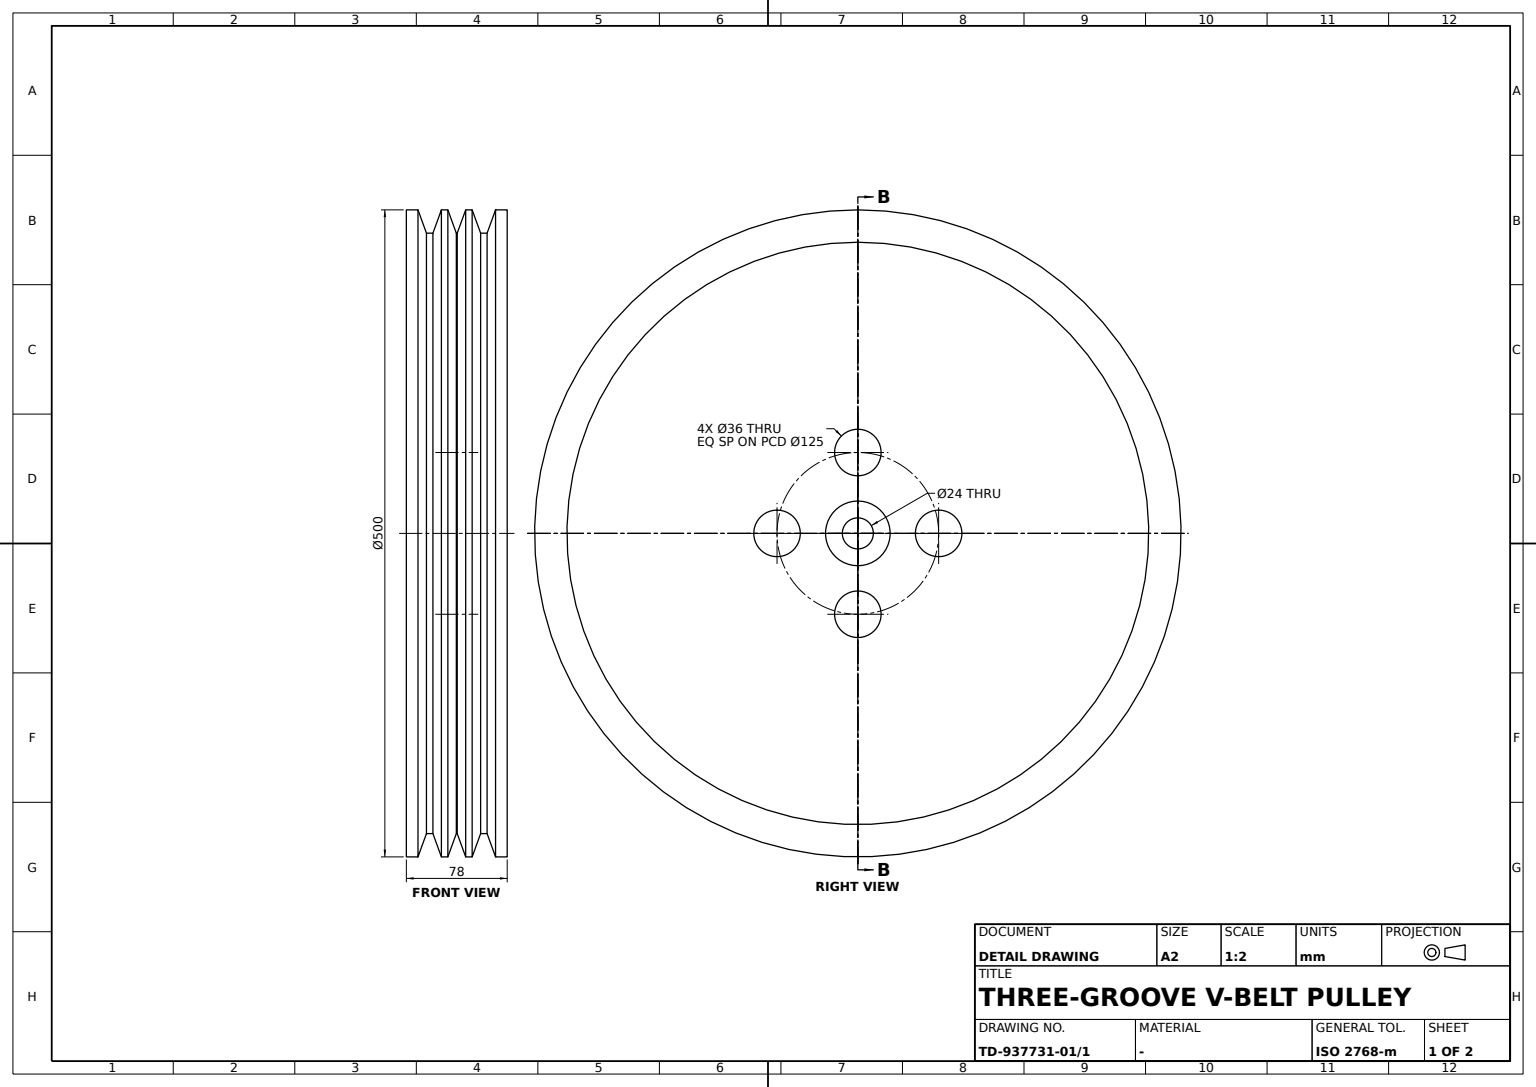
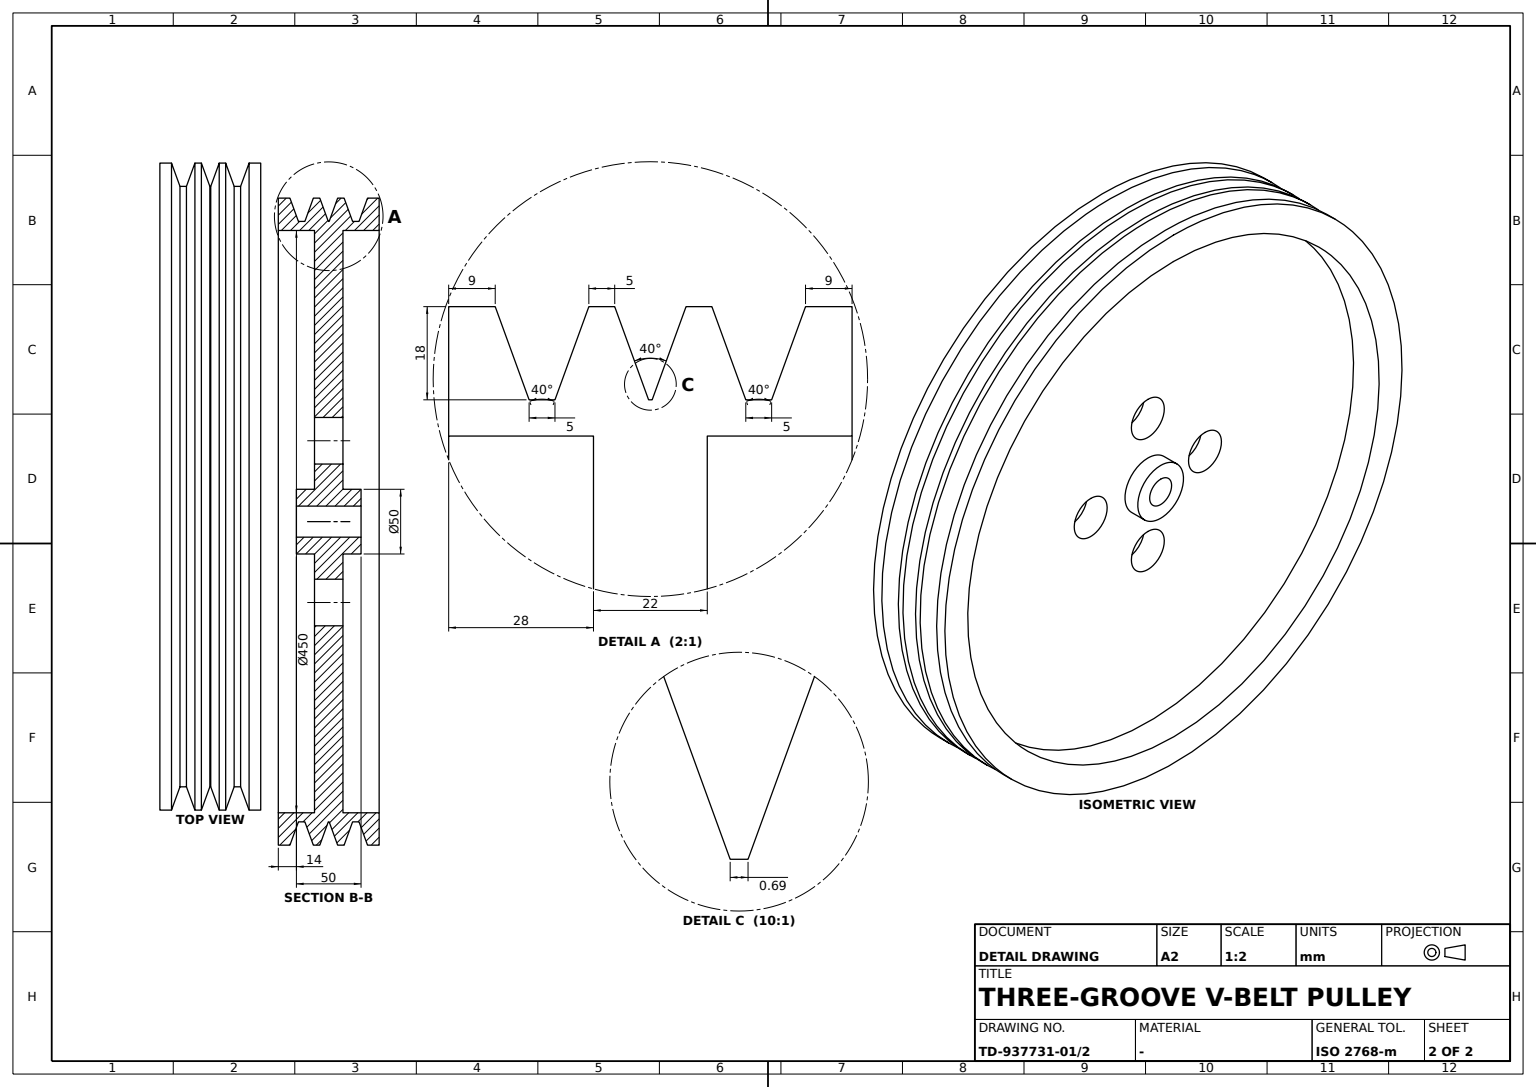
CATIA V5 part; units mm, degrees
sketch "Sketch2" plane through (0, 0, 0) normal (1, 0, 0) x (0, 1, 0)
  point P0 (-30, 250)
  line L0 (-30, 250) -> (-39, 250)
  point P1 (-39, 250)
  line L1 (-39, 250) -> (-39, 225)
  point P2 (-39, 225)
  line L2 (-39, 225) -> (-11, 225)
  point P3 (-11, 225)
  line L3 (-11, 225) -> (-11, 25)
  point P4 (-11, 25)
  line L4 (-11, 25) -> (-25, 25)
  point P5 (-25, 25)
  line L5 (-25, 25) -> (-25, 12)
  point P6 (-25, 12)
  line L6 (-25, 12) -> (0, 12)
  point P7 (0, 12)
  line L7 (-30, 250) -> (-23.4485, 232)
  point P8 (-23.4485, 232)
  line L8 (-23.4485, 232) -> (-18.4485, 232)
  point P9 (-18.4485, 232)
  line L9 (-18.4485, 232) -> (-11.8971, 250)
  point P10 (-11.8971, 250)
  line L10 (-11.8971, 250) -> (-6.8971, 250)
  point P11 (-6.8971, 250)
  line L11 (-6.8971, 250) -> (-0.3456, 232)
  point P12 (-0.3456, 232)
  line L12 (0, 0) -> (0, 340) construction
  line L13 (-0.3456, 232) -> (0, 232)
  point P13 (0, 232)
  point P14 (0, 0)
  point P15 (30, 250)
  point P16 (39, 250)
  point P17 (39, 225)
  point P18 (11, 225)
  point P19 (11, 25)
  point P20 (25, 25)
  point P21 (25, 12)
  point P22 (0, 12)
  point P23 (23.4485, 232)
  point P24 (18.4485, 232)
  point P25 (11.8971, 250)
  point P26 (6.8971, 250)
  point P27 (0.3456, 232)
  point P28 (0, 232)
  line L14 (30, 250) -> (39, 250)
  line L15 (39, 250) -> (39, 225)
  line L16 (39, 225) -> (11, 225)
  line L17 (11, 225) -> (11, 25)
  line L18 (11, 25) -> (25, 25)
  line L19 (25, 25) -> (25, 12)
  line L20 (25, 12) -> (0, 12)
  line L21 (30, 250) -> (23.4485, 232)
  line L22 (23.4485, 232) -> (18.4485, 232)
  line L23 (18.4485, 232) -> (11.8971, 250)
  line L24 (11.8971, 250) -> (6.8971, 250)
  line L25 (6.8971, 250) -> (0.3456, 232)
  line L26 (0.3456, 232) -> (0, 232)
  dimension "distance L6 x axis" = 12
  dimension "distance L4 x axis" = 25
  dimension "distance L3 y axis" = 11
  dimension "distance L5 y axis" = 25
  dimension "distance L0 x axis" = 250
  dimension "distance L1 y axis" = 39
  dimension "length L1" = 25
  dimension "length L8" = 5
  dimension "length L10" = 5
  dimension "angle y axis L11" = 20
  dimension "distance L8 L2" = 7
  dimension "distance L10 L8" = 18
  dimension "angle L7 L9" = 40
  constraint horizontal L0 x-axis
  constraint horizontal L2 x-axis
  constraint horizontal L4 x-axis
  constraint horizontal L6 x-axis
  constraint horizontal L8 x-axis
  constraint horizontal L10 x-axis
  constraint horizontal L13 x-axis
  constraint vertical L1 y-axis
  constraint vertical L3 y-axis
  constraint vertical L5 y-axis
  constraint vertical L12 y-axis
  constraint coincidence P7 y-axis
  constraint coincidence P12 L8
  constraint coincidence P7 P22
  constraint coincidence P13 P28
  constraint parallelism L11 L7
  constraint symmetry origin P14 L12
  constraint symmetry P0 P15 L12
  constraint symmetry P1 P16 L12
  constraint symmetry P2 P17 L12
  constraint symmetry P3 P18 L12
  constraint symmetry P4 P19 L12
  constraint symmetry P5 P20 L12
  constraint symmetry P6 P21 L12
  constraint symmetry P7 P22 L12
  constraint symmetry P8 P23 L12
  constraint symmetry P9 P24 L12
  constraint symmetry P10 P25 L12
  constraint symmetry P11 P26 L12
  constraint symmetry P12 P27 L12
  constraint symmetry P13 P28 L12
  constraint symmetry L0 L14 L12
  constraint symmetry L1 L15 L12
  constraint symmetry L2 L16 L12
  constraint symmetry L3 L17 L12
  constraint symmetry L4 L18 L12
  constraint symmetry L5 L19 L12
  constraint symmetry L6 L20 L12
  constraint symmetry L7 L21 L12
  constraint symmetry L8 L22 L12
  constraint symmetry L9 L23 L12
  constraint symmetry L10 L24 L12
  constraint symmetry L11 L25 L12
  constraint symmetry L13 L26 L12
revolve "Shaft1" add sketch "Sketch2" angle 360 about axis through (0, 0, 0) along (0, 1, 0)
sketch "Sketch3" plane through (0, 11, 0) normal (0, 1, 0) x (-1, 0, 0)
  circle A0 centre (0, 0) radius 62.5 construction
  circle A1 centre (0, 62.5) radius 18
  point P0 (0, 62.5)
  circle A2 centre (62.5, 0) radius 18
  point P1 (62.5, 0)
  circle A3 centre (0, -62.5) radius 18
  point P2 (0, -62.5)
  point P3 (0, -80.5)
  circle A4 centre (-62.5, 0) radius 18
  point P4 (-62.5, 0)
  point P5 (-59.908, -17.8124)
  dimension "radius A0" = 62.5
  dimension "radius A1" = 18
  dimension "radius A2" = 18
  dimension "radius A3" = 18
  dimension "radius A4" = 18
  constraint coincidence P0 A0
  constraint coincidence P0 y-axis
  constraint coincidence P1 A0
  constraint coincidence P1 x-axis
  constraint coincidence P2 A0
  constraint coincidence P2 y-axis
  constraint coincidence A3 P3
  constraint coincidence P3 y-axis
  constraint coincidence P4 A0
  constraint coincidence P4 x-axis
  constraint coincidence A4 P5
  constraint coincidence P5 A0
extrude "Pocket1" cut sketch "Sketch3" against normal blind 87
sketch "Sketch1" plane through (0, 0, 0) normal (1, 0, 0) x (0, 1, 0)
